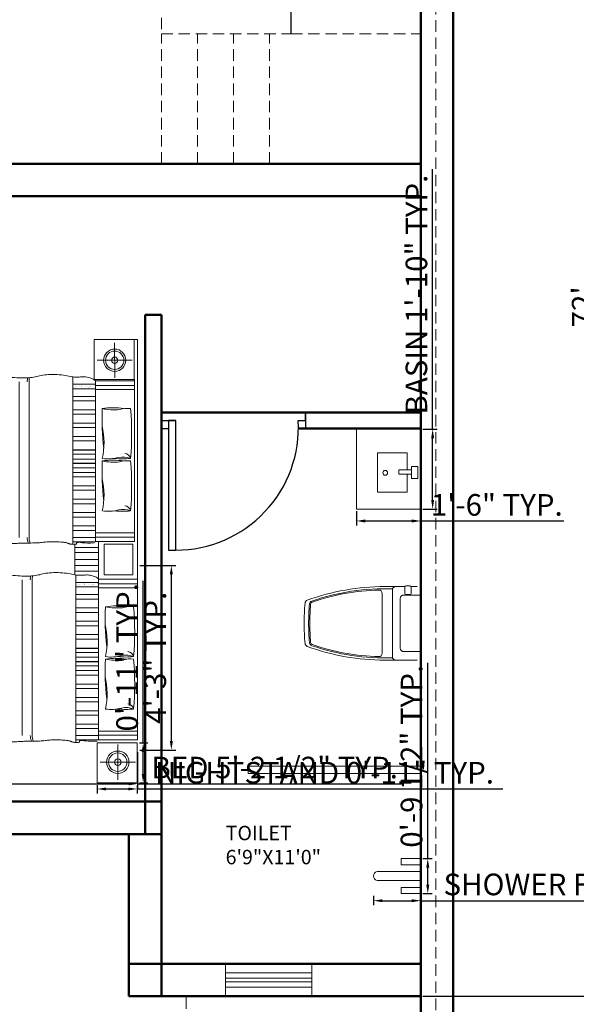
# Model space of a CAD drawing. Units: inches. Extents: x 2123 to 2977, y 1464 to 2698.
# Tile 5 of 10: x 2647 to 2801, y 1923 to 2196. Entities that reach past the tile are written whole.
import ezdxf

# ---------------------------------------------------------------- set-up
doc = ezdxf.new("R2010")
doc.units = ezdxf.units.IN
doc.linetypes.add('HIDDEN2', pattern=[4.7625, 3.175, -1.5875])
for name, color, linetype, lineweight in [('A-ANNO-DIMS', 2, 'Continuous', 18), ('A-AREA-IDEN', 7, 'Continuous', 25), ('A-DOOR', 4, 'Continuous', 25), ('A-FLOR-FIXT', 8, 'Continuous', 20), ('A-FLOR-OVHD', 253, 'HIDDEN2', 18), ('A-FLOR-STRS', 7, 'Continuous', 25), ('A-FLOR-STRS-HIDN', 253, 'HIDDEN2', 18), ('A-FURN', 8, 'Continuous', 18), ('A-FURN-PATT', 252, 'Continuous', 9), ('A-GLAZ', 4, 'Continuous', 18), ('A-WALL', 7, 'Continuous', 50), ('C-PROP', 21, 'HIDDEN2', 18)]:
    doc.layers.add(name, color=color, linetype=linetype, lineweight=lineweight)
doc.styles.get("Standard").update_dxf_attribs({"font": 'arial.ttf'})
doc.dimstyles.new('ISO-25', dxfattribs={"dimtxt": 6, "dimasz": 2.5, "dimexe": 1.25, "dimexo": 0.625, "dimtad": 1, "dimdec": 0, "dimlunit": 3, "dimtxsty": 'Standard', "dimcen": 2.5, "dimadec": 0, "dimazin": 0, "dimtfac": 1, "dimtdec": 0, "dimtmove": 0, "dimatfit": 3, "dimfxl": 1, "dimarcsym": 0})

# ---------------------------------------------------------------- blocks, each defined once
blk = doc.blocks.new('*D9')
at = {"layer": 'A-ANNO-DIMS', "color": 0, "lineweight": -2, "transparency": 16777216}
for p, q in [((2767.56, 2548.37), (2808.58, 2548.37)), ((2807.33, 2545.87), (2807.33, 1686.46)), ((2767.56, 1683.96), (2808.58, 1683.96))]:
    blk.add_line(p, q, dxfattribs=at)
at = {"layer": 'A-ANNO-DIMS', "color": 0, "transparency": 16777216}
for points in [[(2806.91, 2545.87), (2807.74, 2545.87), (2807.33, 2548.37)], [(2806.91, 1686.46), (2807.74, 1686.46), (2807.33, 1683.96)]]:
    blk.add_solid(points, dxfattribs=at)
at = {"layer": 'Defpoints', "color": 0, "transparency": 16777216}
for p in [(2766.94, 2548.37), (2766.94, 1683.96), (2807.33, 1683.96)]:
    blk.add_point(p, dxfattribs=at)
at = {"layer": 'A-ANNO-DIMS', "color": 0, "transparency": 16777216, "insert": (2803.69, 2116.16), "char_height": 6, "attachment_point": 5, "rotation": 90}
blk.add_mtext("72'", dxfattribs=at)
blk = doc.blocks.new('WC-PLAN')
for p, q in [((27.97, 20.42), (22.38, 20.42)), ((24.5, 19.48), (24.5, 10.21)), ((27.93, 20.26), (27.93, 18.53)), ((29.37, 20.57), (28.24, 20.57)), ((31.41, 20.42), (29.65, 20.42)), ((29.69, 20.26), (29.69, 18.53)), ((32.35, 19.48), (32.35, 10.21)), ((21.67, 18.51), (21.67, 10.21)), ((26.7, 17.12), (26.7, 10.21)), ((32.35, 18.06), (27.64, 18.06)), ((29.37, 18.22), (28.24, 18.22)), ((28.24, 18.22), (28.24, 18.06)), ((29.37, 18.22), (29.37, 18.06)), ((21.67, 1.91), (21.67, 10.21)), ((24.5, 0.94), (24.5, 10.21)), ((26.7, 3.3), (26.7, 10.21)), ((32.35, 0.94), (32.35, 10.21)), ((32.35, 2.36), (27.64, 2.36)), ((31.41, 0), (22.38, 0))]:
    blk.add_line(p, q)
for centre, radius, start, end in [((22.38, -42.41), 62.82, 90, 110.0218), ((22.38, -42.41), 62.2, 88.0034, 109.0034), ((22.38, -42.41), 61.88, 91.5459, 109.0034), ((20.73, 18.51), 0.942, 0, 91.5459), ((25.44, 19.48), 0.942, 90, 180), ((28.24, 20.26), 0.314, 150, 180), ((28.24, 20.26), 0.314, 90, 150), ((29.37, 20.26), 0.314, 30, 90), ((29.37, 20.26), 0.314, 0, 30), ((1.19, 15.74), 0.942, 110.0218, 174.8892), ((2.43, 15.51), 0.942, 109.0034, 174.9977), ((27.64, 17.12), 0.942, 90, 180), ((28.24, 18.53), 0.314, 180, 270), ((29.37, 18.53), 0.314, 270, 0), ((62.98, 10.21), 62.98, 174.8892, 180), ((62.98, 10.21), 61.73, 174.9977, 180), ((62.98, 10.21), 61.41, 174.9977, 180), ((2.43, 15.51), 0.628, 109.0034, 174.9977), ((62.98, 10.21), 62.98, 180, 185.1108), ((62.98, 10.21), 61.73, 180, 185.0023), ((62.98, 10.21), 61.41, 180, 185.0023), ((1.19, 4.68), 0.942, 185.1108, 249.9782), ((22.38, 62.82), 62.82, 249.9782, 270), ((2.43, 4.91), 0.942, 185.0023, 250.9966), ((2.43, 4.91), 0.628, 185.0023, 250.9966), ((22.38, 62.82), 62.2, 250.9966, 271.9966), ((22.38, 62.82), 61.88, 250.9966, 268.4541), ((27.64, 3.3), 0.942, 180, 270), ((20.73, 1.91), 0.942, 268.4541, 0), ((25.44, 0.94), 0.942, 180, 270)]:
    blk.add_arc(centre, radius, start, end)
blk = doc.blocks.new('VANITY-BASIN')
blk.add_line((14.09, 15.62), (5.85, 15.62))
for points in [[(0, 22.13), (17.86, 22.13), (17.86, 0), (0, 0)], [(15.3, 11.79), (17.03, 11.79), (17.03, 8.46), (15.3, 8.46)]]:
    blk.add_lwpolyline(points, close=True)
for points in [[(14.09, 9.69), (14.09, 4.64), (5.85, 4.64), (5.85, 15.62)], [(14.09, 15.62), (14.09, 10.87)], [(15.3, 9.69), (11.78, 9.69), (11.78, 10.87), (15.3, 10.87)]]:
    blk.add_lwpolyline(points)
blk.add_circle((8.01, 10.03), 0.665)
blk = doc.blocks.new('SHOWER-FITTING')
for points in [[(7.7, 9.7), (13.11, 9.7), (13.11, 7.96), (7.7, 7.96)], [(7.7, 1.74), (13.11, 1.74), (13.11, 0), (7.7, 0)]]:
    blk.add_lwpolyline(points, close=True)
blk.add_lwpolyline([(1, 6.13), (13.11, 6.13), (13.11, 3.63), (1, 3.63)])
blk.add_arc((1.29, 4.88), 1.29, 102.8146, 257.1854)
blk = doc.blocks.new('BED-WITH-PILLOWS')
for p, q in [((5.75, 4.05), (5.75, 47.2)), ((6.24, 4.05), (6.24, 47.2)), ((10.69, 4.05), (10.69, 47.2)), ((11.18, 4.05), (11.18, 47.2)), ((15.63, 4.05), (15.63, 47.2)), ((16.12, 4.05), (16.12, 47.2)), ((25.45, 4.05), (25.45, 47.2)), ((25.94, 4.05), (25.94, 47.2)), ((30.39, 4.05), (30.39, 47.2)), ((33.11, 4.05), (33.11, 47.2)), ((45.27, 2.11), (45.27, 48.58)), ((51.57, 46.51), (45.27, 46.51)), ((51.57, 45.27), (45.27, 45.27)), ((62.41, 46.17), (51.57, 46.17)), ((62.41, 45.03), (51.57, 45.03)), ((51.57, 28.22), (45.27, 28.22)), ((62.41, 5.26), (51.57, 5.26)), ((62.41, 4.13), (51.57, 4.13)), ((62.41, 2.86), (51.57, 2.86))]:
    blk.add_line(p, q)
for points in [[(51.2, 2.51), (50.14, 2.47), (49.31, 2.46), (48.67, 2.48), (48.19, 2.52), (47.84, 2.56), (47.58, 2.61), (47.39, 2.66), (47.22, 2.69), (47.07, 2.7), (46.91, 2.7), (46.77, 2.68), (46.63, 2.65), (46.51, 2.61), (46.41, 2.56), (46.33, 2.52), (46.28, 2.47), (46.26, 2.42), (46.26, 2.38), (46.28, 2.35), (46.3, 2.31), (46.32, 2.28), (46.32, 2.25), (46.31, 2.22), (46.27, 2.2), (46.19, 2.17), (46.08, 2.15), (45.94, 2.13), (45.78, 2.12), (45.61, 2.11), (45.43, 2.1), (45.25, 2.11), (45.07, 2.12), (44.89, 2.14), (44.73, 2.16), (44.57, 2.2), (44.42, 2.24), (44.28, 2.28), (44.15, 2.32), (44.02, 2.37), (43.89, 2.41), (43.77, 2.46), (43.65, 2.5), (43.51, 2.54), (43.35, 2.58), (43.16, 2.62), (42.93, 2.66), (42.65, 2.69), (42.31, 2.72), (41.91, 2.75), (41.46, 2.78), (40.97, 2.8), (40.46, 2.82), (39.94, 2.82), (39.43, 2.83), (38.94, 2.82), (38.48, 2.81), (38.08, 2.78), (37.71, 2.75), (37.37, 2.71), (37.04, 2.67), (36.71, 2.63), (36.37, 2.59), (36, 2.55), (35.6, 2.52), (35.14, 2.5), (34.65, 2.49), (34.14, 2.48), (33.61, 2.47), (33.1, 2.47), (32.6, 2.47), (32.14, 2.47), (31.72, 2.47), (31.37, 2.46), (31.06, 2.45), (30.79, 2.44), (30.55, 2.42), (30.31, 2.41), (30.08, 2.39), (29.82, 2.38), (29.54, 2.36), (29.21, 2.35), (28.86, 2.33), (28.48, 2.32), (28.09, 2.31), (27.69, 2.3), (27.3, 2.29), (26.93, 2.28), (26.58, 2.27), (26.27, 2.26), (25.99, 2.25), (25.73, 2.24), (25.49, 2.24), (25.25, 2.25), (25.02, 2.27), (24.78, 2.29), (24.53, 2.33), (24.27, 2.38), (23.99, 2.44), (23.7, 2.51), (23.41, 2.57), (23.12, 2.62), (22.85, 2.66), (22.59, 2.69), (22.35, 2.68), (22.13, 2.65), (17.06, 2.6), (16.88, 2.53), (16.71, 2.44), (16.54, 2.35), (16.37, 2.25), (16.2, 2.15), (16.01, 2.05), (15.8, 1.96), (15.58, 1.89), (15.34, 1.82), (15.08, 1.77), (14.81, 1.72), (14.53, 1.69), (14.24, 1.67), (13.93, 1.66), (13.62, 1.66), (13.3, 1.67), (12.98, 1.69), (12.67, 1.72), (12.35, 1.75), (12.05, 1.79), (11.76, 1.84), (11.49, 1.89), (11.24, 1.94), (11, 1.99), (10.76, 2.04), (10.52, 2.09), (10.28, 2.14), (10.02, 2.18), (9.74, 2.21), (9.43, 2.24), (9.08, 2.25), (8.71, 2.26), (8.32, 2.26), (7.93, 2.25), (7.53, 2.24), (7.16, 2.22), (6.8, 2.2), (6.49, 2.17), (6.21, 2.15), (5.97, 2.12), (5.77, 2.09), (5.59, 2.06), (5.44, 2.03), (5.3, 2), (5.18, 1.97), (5.07, 1.94), (4.96, 1.91), (4.85, 1.88), (4.74, 1.85), (4.63, 1.81), (4.51, 1.77), (4.39, 1.72), (4.26, 1.67), (4.12, 1.61), (3.98, 1.53), (3.82, 1.46), (3.67, 1.37), (3.51, 1.27), (3.35, 1.17), (3.19, 1.06), (3.04, 0.94), (2.9, 0.81), (2.76, 0.68), (2.64, 0.54), (2.52, 0.41), (2.4, 0.28), (2.28, 0.18), (2.15, 0.09), (2, 0.03), (1.84, 0), (1.67, 0.01), (1.48, 0.05), (1.28, 0.12), (1.09, 0.21), (0.89, 0.33), (0.71, 0.46), (0.54, 0.6), (0.39, 0.74), (0.26, 0.89), (0.17, 1.04), (0.09, 1.19), (0.04, 1.34), (0.01, 1.49), (0, 1.65), (0.01, 1.81), (0.04, 1.97), (0.08, 2.13), (0.14, 2.3), (0.21, 2.47), (0.29, 2.64), (0.38, 2.82), (0.48, 3), (0.58, 3.18), (0.68, 3.37), (0.79, 3.57), (0.9, 3.77), (1, 3.97), (1.09, 4.19), (1.18, 4.41), (1.26, 4.64), (1.32, 4.89), (1.37, 5.14), (1.4, 5.4), (1.42, 5.68), (1.43, 5.97), (1.43, 6.29), (1.42, 6.62), (1.42, 6.98), (1.41, 7.36), (1.41, 7.77), (1.42, 8.21), (1.44, 8.67), (1.46, 9.16), (1.49, 9.65), (1.52, 10.16), (1.55, 10.68), (1.58, 11.19), (1.61, 11.69), (1.64, 12.19), (1.67, 12.67), (1.69, 13.14), (1.72, 13.6), (1.73, 14.05), (1.75, 14.49), (1.77, 14.91), (1.78, 15.32), (1.79, 15.72), (1.79, 16.1), (1.8, 16.48), (1.81, 16.85), (1.83, 17.21), (1.85, 17.56), (1.88, 17.91), (1.91, 18.25), (1.96, 18.58), (2.01, 18.93), (2.07, 19.29), (2.14, 19.68), (2.21, 20.11), (2.29, 20.58), (2.36, 21.11), (2.44, 21.71), (2.51, 22.39), (2.58, 23.13), (2.64, 23.92), (2.69, 24.77), (2.72, 25.64), (2.73, 26.54), (2.71, 27.44), (2.67, 28.35), (2.59, 24.41), (2.49, 25.28), (2.37, 26.12), (2.24, 26.93), (2.11, 27.7), (1.98, 28.42), (1.86, 29.08), (1.76, 29.68), (1.69, 30.2), (1.64, 30.67), (1.61, 31.08), (1.59, 31.44), (1.59, 31.77), (1.6, 32.08), (1.61, 32.36), (1.63, 32.64), (1.64, 32.92), (1.66, 33.21), (1.67, 33.51), (1.67, 33.82), (1.68, 34.16), (1.68, 34.52), (1.68, 34.92), (1.67, 35.35), (1.66, 35.83), (1.64, 36.35), (1.62, 36.91), (1.61, 37.51), (1.6, 38.16), (1.59, 38.85), (1.59, 39.57), (1.6, 40.34), (1.62, 41.15), (1.65, 41.98), (1.68, 42.82), (1.7, 43.65), (1.72, 44.46), (1.73, 45.24), (1.72, 45.95), (1.7, 46.6), (1.64, 47.17), (1.57, 47.65), (1.48, 48.08), (1.39, 48.45), (1.29, 48.77), (1.19, 49.06), (1.1, 49.32), (1.02, 49.57), (0.96, 49.81), (0.91, 50.04), (0.89, 50.26), (0.87, 50.46), (0.88, 50.65), (0.9, 50.81), (0.93, 50.95), (0.98, 51.06), (1.04, 51.14), (1.12, 51.2), (1.21, 51.22), (1.31, 51.22), (1.43, 51.19), (1.55, 51.15), (1.69, 51.09), (1.84, 51.01), (2.01, 50.92), (2.18, 50.81), (2.36, 50.7), (2.54, 50.57), (2.72, 50.45), (2.91, 50.31), (3.09, 50.18), (3.27, 50.04), (3.45, 49.9), (3.62, 49.77), (3.78, 49.63), (3.93, 49.5), (4.08, 49.37), (4.23, 49.24), (4.37, 49.11), (4.5, 48.99), (4.63, 48.86), (4.76, 48.74), (4.88, 48.62), (5.01, 48.5), (5.14, 48.4), (5.27, 48.3), (5.41, 48.2), (5.55, 48.12), (5.71, 48.05), (5.87, 48), (6.04, 47.95), (6.22, 47.92), (6.39, 47.9), (6.56, 47.89), (6.73, 47.9), (6.89, 47.92), (7.04, 47.96), (7.18, 48.01), (7.31, 48.07), (7.43, 48.13), (7.53, 48.2), (7.61, 48.27), (7.67, 48.33), (7.71, 48.39), (7.73, 48.44), (7.73, 48.49), (7.71, 48.52), (7.68, 48.55), (7.63, 48.58), (7.56, 48.6), (7.49, 48.61), (7.42, 48.62), (7.33, 48.63), (7.25, 48.64), (7.16, 48.64), (7.07, 48.64), (6.99, 48.63), (6.91, 48.62), (6.83, 48.6), (6.77, 48.58), (6.71, 48.55), (6.67, 48.52), (6.63, 48.5), (6.6, 48.47), (6.57, 48.46), (6.56, 48.46), (6.55, 48.48), (6.54, 48.51), (6.54, 48.58)], [(6.54, 48.66), (6.54, 48.76), (6.55, 48.86), (6.56, 48.97), (6.58, 49.08), (6.61, 49.18), (6.63, 49.27), (6.67, 49.34), (6.7, 49.4), (6.75, 49.44), (6.79, 49.47), (6.84, 49.5), (6.9, 49.51), (6.95, 49.52), (7.01, 49.53), (7.07, 49.53), (7.14, 49.53), (7.21, 49.53), (7.28, 49.53), (7.35, 49.53), (7.43, 49.52), (7.51, 49.5), (7.59, 49.49), (7.68, 49.46), (7.77, 49.43), (7.86, 49.4), (7.96, 49.36), (8.06, 49.31), (8.16, 49.26), (8.27, 49.19), (8.37, 49.12), (8.48, 49.04), (8.59, 48.95), (8.69, 48.86), (8.8, 48.76), (8.9, 48.66), (9.01, 48.56), (9.1, 48.45), (9.2, 48.35), (9.29, 48.25), (9.38, 48.16), (9.48, 48.07), (9.61, 48), (9.76, 47.94), (9.95, 47.91), (10.18, 47.89), (10.46, 47.89), (10.81, 47.93), (11.21, 47.98), (11.65, 48.06), (12.15, 48.14), (12.68, 48.23), (13.25, 48.32), (13.84, 48.41), (14.46, 48.49), (15.09, 48.55), (15.74, 48.6), (16.41, 48.64), (17.08, 48.66), (22.63, 48.67), (23.31, 48.67), (23.98, 48.66), (24.65, 48.64), (25.32, 48.61), (25.97, 48.57), (26.62, 48.53), (27.26, 48.49), (27.89, 48.44), (28.51, 48.4), (29.12, 48.36), (29.71, 48.33), (30.3, 48.3), (30.87, 48.28), (31.43, 48.27), (31.97, 48.28), (32.5, 48.29), (33, 48.32), (33.49, 48.36), (33.95, 48.42), (34.39, 48.49), (34.81, 48.58), (35.23, 48.67), (35.64, 48.77), (36.07, 48.87), (36.5, 48.96), (36.96, 49.05), (37.46, 49.12), (37.99, 49.18), (38.55, 49.22), (39.13, 49.24), (39.73, 49.25), (40.33, 49.24), (40.93, 49.22), (41.52, 49.18), (42.1, 49.12), (42.65, 49.05), (43.17, 48.96), (43.66, 48.87), (44.14, 48.78), (44.58, 48.7), (45, 48.62), (45.4, 48.56), (45.77, 48.51), (46.12, 48.5), (46.45, 48.5), (46.77, 48.51), (47.08, 48.53), (47.4, 48.56), (47.73, 48.57), (48.08, 48.58), (48.45, 48.58), (48.84, 48.55), (49.25, 48.49), (49.68, 48.41), (50.1, 48.3), (50.5, 48.16), (50.88, 47.98), (51.23, 47.77), (51.53, 47.52)], [(51.57, 47.43), (51.57, 2.81), (45.27, 2.81)], [(51.57, 47.43), (62.41, 47.43)], [(45.27, 43.15), (51.57, 43.15)], [(51.57, 41.91), (45.27, 41.91)], [(45.27, 39.44), (51.57, 39.44)], [(51.57, 38.2), (45.27, 38.2)], [(45.27, 35.73), (51.57, 35.73)], [(51.57, 34.5), (45.27, 34.5)], [(45.27, 32.03), (51.57, 32.03)], [(51.57, 30.79), (45.27, 30.79)], [(45.27, 28.32), (51.57, 28.32)], [(51.57, 27.09), (45.27, 27.09)], [(45.27, 25.74), (51.57, 25.74)], [(45.27, 24.62), (51.57, 24.62)], [(51.57, 24.51), (45.27, 24.51)], [(51.57, 23.38), (45.27, 23.38)], [(45.27, 22.04), (51.57, 22.04)], [(51.57, 20.8), (45.27, 20.8)], [(45.27, 18.33), (51.57, 18.33)], [(51.57, 17.1), (45.27, 17.1)], [(45.27, 14.63), (51.57, 14.63)], [(51.57, 13.39), (45.27, 13.39)], [(45.27, 10.92), (51.57, 10.92)], [(51.57, 9.69), (45.27, 9.69)], [(45.27, 7.22), (51.57, 7.22)], [(51.57, 5.98), (45.27, 5.98)], [(45.27, 4.05), (51.57, 4.05)]]:
    blk.add_lwpolyline(points)
blk.add_lwpolyline([(51.57, 46.51), (51.57, 45.27), (45.27, 45.27), (45.27, 46.51)], close=True)
for centre, radius, start, end in [((9.74, 47.23), 3.5, 168.8455, 180.4575), ((14.19, 47.23), 3.5, 168.5644, 180.4575), ((14.68, 47.23), 3.5, 167.3874, 180.4575), ((19.13, 47.23), 3.5, 156.778, 180.4575), ((19.62, 47.23), 3.5, 156.3002, 180.4575), ((28.95, 47.23), 3.5, 157.2176, 180.4575), ((29.45, 47.23), 3.5, 157.7219, 180.4575), ((36.12, 47.23), 3.5, 162.3249, 180.4575), ((36.61, 47.23), 3.5, 162.5343, 180.4575), ((113.8, 36.55), 60.42, 176.9417, 187.4263), ((56.43, 21.05), 18.95, 81.0114, 98.9886), ((56.69, 54.69), 15.26, 257.8171, 275.8068), ((60.35, 32.94), 6.89, 82.0225, 107.8578), ((-19.09, 32.85), 80.7, 355.082, 4.918), ((33.93, 30.3), 20.02, 347.406, 13.4182), ((59.54, 25.52), 1.81, 13.0862, 85.1007), ((113.8, 22.01), 60.42, 176.9417, 187.4263), ((55.08, 36.57), 10.76, 261.3968, 285.5408), ((56.43, 6.52), 18.95, 81.0114, 98.9886), ((56.69, 40.15), 15.26, 257.8171, 275.8068), ((59.11, 48.58), 22.76, 264.4677, 275.5323), ((59.18, 20.45), 5.88, 68.7829, 101.9106), ((60.35, 18.41), 6.89, 82.0225, 107.8578), ((-19.09, 18.32), 80.7, 355.082, 4.918), ((33.93, 15.76), 20.02, 347.406, 13.4182), ((55.08, 22.03), 10.76, 261.3968, 285.5408), ((59.11, 34.05), 22.76, 264.4677, 275.5323), ((59.18, 5.91), 5.88, 68.7829, 101.9106), ((59.54, 10.99), 1.81, 13.0862, 85.1007), ((14.19, 4.02), 3.5, 179.5425, 217.0761), ((14.68, 4.02), 3.5, 179.5425, 219.1707), ((19.13, 4.02), 3.5, 179.5425, 212.5319), ((19.62, 4.02), 3.5, 179.5425, 208.4654), ((28.95, 4.02), 3.5, 179.5425, 210.3906), ((29.45, 4.02), 3.5, 179.5425, 210.1306), ((36.12, 4.02), 3.5, 179.5425, 206.8424), ((36.61, 4.02), 3.5, 179.5425, 206.471)]:
    blk.add_arc(centre, radius, start, end)
blk = doc.blocks.new('NIGHTSTAND-WITH-LAMP')
for p, q in [((5.74, 10.64), (5.72, 0.88)), ((0.85, 5.76), (10.61, 5.76))]:
    blk.add_line(p, q)
blk.add_lwpolyline([(11.12, 0), (11.12, 11.12), (0, 11.12), (0, 0)], close=True)
for radius in [3.1, 2.55, 0.89]:
    blk.add_circle((5.73, 5.76), radius)
blk = doc.blocks.new('SHOWER-SCREEN')
for p, q in [((47.94, 2), (0, 2)), ((0, 2), (0, 0)), ((0, 0), (47.94, 0))]:
    blk.add_line(p, q)
blk = doc.blocks.new('*D36')
at = {"layer": 'A-ANNO-DIMS', "color": 0, "lineweight": -2, "transparency": 16777216}
for p, q in [((2761.26, 2082.2), (2761.26, 2154.4)), ((2758.56, 2082.2), (2762.51, 2082.2)), ((2761.26, 2062.56), (2761.26, 2079.7)), ((2758.56, 2060.06), (2762.51, 2060.06))]:
    blk.add_line(p, q, dxfattribs=at)
at = {"layer": 'A-ANNO-DIMS', "color": 0, "transparency": 16777216}
for points in [[(2760.84, 2079.7), (2761.67, 2079.7), (2761.26, 2082.2)], [(2760.84, 2062.56), (2761.67, 2062.56), (2761.26, 2060.06)]]:
    blk.add_solid(points, dxfattribs=at)
at = {"layer": 'Defpoints', "color": 0, "transparency": 16777216}
for p in [(2757.94, 2082.2), (2761.26, 2082.2), (2757.94, 2060.06)]:
    blk.add_point(p, dxfattribs=at)
at = {"layer": 'A-ANNO-DIMS', "color": 0, "transparency": 16777216, "insert": (2757.53, 2119.55), "char_height": 6, "attachment_point": 5, "rotation": 90}
blk.add_mtext('BASIN 1\'-10" TYP.', dxfattribs=at)
blk = doc.blocks.new('*D37')
at = {"layer": 'A-ANNO-DIMS', "color": 0, "lineweight": -2, "transparency": 16777216}
for p, q in [((2740.08, 2059.44), (2740.08, 2055.49)), ((2757.94, 2059.44), (2757.94, 2055.49)), ((2742.58, 2056.74), (2755.44, 2056.74)), ((2757.94, 2056.74), (2797.69, 2056.74))]:
    blk.add_line(p, q, dxfattribs=at)
at = {"layer": 'A-ANNO-DIMS', "color": 0, "transparency": 16777216}
for points in [[(2742.58, 2057.16), (2742.58, 2056.32), (2740.08, 2056.74)], [(2755.44, 2057.16), (2755.44, 2056.32), (2757.94, 2056.74)]]:
    blk.add_solid(points, dxfattribs=at)
at = {"layer": 'Defpoints', "color": 0, "transparency": 16777216}
for p in [(2740.08, 2060.06), (2757.94, 2060.06), (2757.94, 2056.74)]:
    blk.add_point(p, dxfattribs=at)
at = {"layer": 'A-ANNO-DIMS', "color": 0, "transparency": 16777216, "insert": (2779.06, 2060.43), "char_height": 6, "attachment_point": 5}
blk.add_mtext('1\'-6" TYP.', dxfattribs=at)
blk = doc.blocks.new('*D44')
at = {"layer": 'A-ANNO-DIMS', "color": 0, "lineweight": -2, "transparency": 16777216}
for p, q in [((2744.82, 1952.72), (2744.82, 1950.13)), ((2747.32, 1951.38), (2755.44, 1951.38)), ((2757.94, 1952.72), (2757.94, 1950.13)), ((2757.94, 1951.38), (2873.2, 1951.38))]:
    blk.add_line(p, q, dxfattribs=at)
at = {"layer": 'A-ANNO-DIMS', "color": 0, "transparency": 16777216}
for points in [[(2747.32, 1951.79), (2747.32, 1950.96), (2744.82, 1951.38)], [(2755.44, 1951.79), (2755.44, 1950.96), (2757.94, 1951.38)]]:
    blk.add_solid(points, dxfattribs=at)
at = {"layer": 'Defpoints', "color": 0, "transparency": 16777216}
for p in [(2744.82, 1953.34), (2757.94, 1953.34), (2757.94, 1951.38)]:
    blk.add_point(p, dxfattribs=at)
at = {"layer": 'A-ANNO-DIMS', "color": 0, "transparency": 16777216, "insert": (2816.82, 1955.11), "char_height": 6, "attachment_point": 5}
blk.add_mtext('SHOWER FITTING 1\'-1" TYP.', dxfattribs=at)
blk = doc.blocks.new('*D45')
at = {"layer": 'A-ANNO-DIMS', "color": 0, "lineweight": -2, "transparency": 16777216}
for p, q in [((2759.9, 1963.04), (2759.9, 2017.35)), ((2758.56, 1963.04), (2761.15, 1963.04)), ((2759.9, 1955.84), (2759.9, 1960.54)), ((2758.56, 1953.34), (2761.15, 1953.34))]:
    blk.add_line(p, q, dxfattribs=at)
at = {"layer": 'A-ANNO-DIMS', "color": 0, "transparency": 16777216}
for points in [[(2759.49, 1960.54), (2760.32, 1960.54), (2759.9, 1963.04)], [(2759.49, 1955.84), (2760.32, 1955.84), (2759.9, 1953.34)]]:
    blk.add_solid(points, dxfattribs=at)
at = {"layer": 'Defpoints', "color": 0, "transparency": 16777216}
for p in [(2757.94, 1963.04), (2759.9, 1963.04), (2757.94, 1953.34)]:
    blk.add_point(p, dxfattribs=at)
at = {"layer": 'A-ANNO-DIMS', "color": 0, "transparency": 16777216, "insert": (2756.17, 1991.45), "char_height": 6, "attachment_point": 5, "rotation": 90}
blk.add_mtext('0\'-9 1/2" TYP.', dxfattribs=at)
blk = doc.blocks.new('*D48')
at = {"layer": 'A-ANNO-DIMS', "color": 0, "lineweight": -2, "transparency": 16777216}
for p, q in [((2616.93, 1992.55), (2616.93, 1982.56)), ((2679.35, 1992.55), (2679.35, 1982.56)), ((2619.43, 1983.81), (2676.85, 1983.81)), ((2679.35, 1983.81), (2752.95, 1983.81))]:
    blk.add_line(p, q, dxfattribs=at)
at = {"layer": 'A-ANNO-DIMS', "color": 0, "transparency": 16777216}
for points in [[(2619.43, 1984.23), (2619.43, 1983.39), (2616.93, 1983.81)], [(2676.85, 1984.23), (2676.85, 1983.39), (2679.35, 1983.81)]]:
    blk.add_solid(points, dxfattribs=at)
at = {"layer": 'Defpoints', "color": 0, "transparency": 16777216}
for p in [(2616.93, 1993.17), (2679.35, 1993.17), (2679.35, 1983.81)]:
    blk.add_point(p, dxfattribs=at)
at = {"layer": 'A-ANNO-DIMS', "color": 0, "transparency": 16777216, "insert": (2717.4, 1987.54), "char_height": 6, "attachment_point": 5}
blk.add_mtext('BED 5\'-2 1/2" TYP.', dxfattribs=at)
blk = doc.blocks.new('*D49')
at = {"layer": 'A-ANNO-DIMS', "color": 0, "lineweight": -2, "transparency": 16777216}
for p, q in [((2679.97, 2044.39), (2689.96, 2044.39)), ((2688.71, 1995.67), (2688.71, 2041.89)), ((2679.97, 1993.17), (2689.96, 1993.17))]:
    blk.add_line(p, q, dxfattribs=at)
at = {"layer": 'A-ANNO-DIMS', "color": 0, "transparency": 16777216}
for points in [[(2688.29, 2041.89), (2689.13, 2041.89), (2688.71, 2044.39)], [(2688.29, 1995.67), (2689.13, 1995.67), (2688.71, 1993.17)]]:
    blk.add_solid(points, dxfattribs=at)
at = {"layer": 'Defpoints', "color": 0, "transparency": 16777216}
for p in [(2679.35, 2044.39), (2688.71, 2044.39), (2679.35, 1993.17)]:
    blk.add_point(p, dxfattribs=at)
at = {"layer": 'A-ANNO-DIMS', "color": 0, "transparency": 16777216, "insert": (2685.02, 2018.78), "char_height": 6, "attachment_point": 5, "rotation": 90}
blk.add_mtext('4\'-3" TYP.', dxfattribs=at)
blk = doc.blocks.new('*D50')
at = {"layer": 'A-ANNO-DIMS', "color": 0, "lineweight": -2, "transparency": 16777216}
for p, q in [((2668.11, 1983.42), (2668.11, 1981.13)), ((2670.61, 1982.38), (2676.73, 1982.38)), ((2679.23, 1983.42), (2679.23, 1981.13)), ((2679.23, 1982.38), (2780.73, 1982.38))]:
    blk.add_line(p, q, dxfattribs=at)
at = {"layer": 'A-ANNO-DIMS', "color": 0, "transparency": 16777216}
for points in [[(2670.61, 1982.8), (2670.61, 1981.96), (2668.11, 1982.38)], [(2676.73, 1982.8), (2676.73, 1981.96), (2679.23, 1982.38)]]:
    blk.add_solid(points, dxfattribs=at)
at = {"layer": 'Defpoints', "color": 0, "transparency": 16777216}
for p in [(2668.11, 1984.05), (2679.23, 1984.05), (2679.23, 1982.38)]:
    blk.add_point(p, dxfattribs=at)
at = {"layer": 'A-ANNO-DIMS', "color": 0, "transparency": 16777216, "insert": (2731.23, 1986.11), "char_height": 6, "attachment_point": 5}
blk.add_mtext('NIGHTSTAND 0\'-11" TYP.', dxfattribs=at)
blk = doc.blocks.new('*D51')
at = {"layer": 'A-ANNO-DIMS', "color": 0, "lineweight": -2, "transparency": 16777216}
for p, q in [((2680.89, 1995.17), (2680.89, 2040.15)), ((2679.85, 1995.17), (2682.14, 1995.17)), ((2680.89, 1986.55), (2680.89, 1992.67)), ((2679.85, 1984.05), (2682.14, 1984.05))]:
    blk.add_line(p, q, dxfattribs=at)
at = {"layer": 'A-ANNO-DIMS', "color": 0, "transparency": 16777216}
for points in [[(2680.48, 1992.67), (2681.31, 1992.67), (2680.89, 1995.17)], [(2680.48, 1986.55), (2681.31, 1986.55), (2680.89, 1984.05)]]:
    blk.add_solid(points, dxfattribs=at)
at = {"layer": 'Defpoints', "color": 0, "transparency": 16777216}
for p in [(2679.23, 1995.17), (2680.89, 1995.17), (2679.23, 1984.05)]:
    blk.add_point(p, dxfattribs=at)
at = {"layer": 'A-ANNO-DIMS', "color": 0, "transparency": 16777216, "insert": (2677.2, 2018.91), "char_height": 6, "attachment_point": 5, "rotation": 90}
blk.add_mtext('0\'-11" TYP.', dxfattribs=at)
blk = doc.blocks.new('*D55')
at = {"layer": 'A-ANNO-DIMS', "color": 0, "lineweight": -2, "transparency": 16777216}
for p, q in [((2758.56, 1924.87), (2820.89, 1924.87)), ((2819.64, 1695.76), (2819.64, 1922.37)), ((2758.56, 1693.26), (2820.89, 1693.26))]:
    blk.add_line(p, q, dxfattribs=at)
at = {"layer": 'A-ANNO-DIMS', "color": 0, "transparency": 16777216}
for points in [[(2819.22, 1922.37), (2820.05, 1922.37), (2819.64, 1924.87)], [(2819.22, 1695.76), (2820.05, 1695.76), (2819.64, 1693.26)]]:
    blk.add_solid(points, dxfattribs=at)
at = {"layer": 'Defpoints', "color": 0, "transparency": 16777216}
for p in [(2757.94, 1924.87), (2819.64, 1924.87), (2757.94, 1693.26)]:
    blk.add_point(p, dxfattribs=at)
at = {"layer": 'A-ANNO-DIMS', "color": 0, "transparency": 16777216, "insert": (2815.91, 1809.06), "char_height": 6, "attachment_point": 5, "rotation": 90}
blk.add_mtext('19\'-3 1/2"', dxfattribs=at)
blk = doc.blocks.new('*D57')
at = {"layer": 'A-ANNO-DIMS', "color": 0, "lineweight": -2, "transparency": 16777216}
for p, q in [((2555.89, 1805.13), (2555.89, 2606.82)), ((2757.94, 1805.13), (2757.94, 2606.82)), ((2558.39, 2605.57), (2755.44, 2605.57))]:
    blk.add_line(p, q, dxfattribs=at)
at = {"layer": 'A-ANNO-DIMS', "color": 0, "transparency": 16777216}
for points in [[(2558.39, 2605.99), (2558.39, 2605.15), (2555.89, 2605.57)], [(2755.44, 2605.99), (2755.44, 2605.15), (2757.94, 2605.57)]]:
    blk.add_solid(points, dxfattribs=at)
at = {"layer": 'Defpoints', "color": 0, "transparency": 16777216}
for p in [(2757.94, 2605.57), (2555.89, 1804.5), (2757.94, 1804.5)]:
    blk.add_point(p, dxfattribs=at)
at = {"layer": 'A-ANNO-DIMS', "color": 0, "transparency": 16777216, "insert": (2656.91, 2609.26), "char_height": 6, "attachment_point": 5}
blk.add_mtext('16\'-10"', dxfattribs=at)

msp = doc.modelspace()

# ---------------------------------------------------------------- hatches: boundary and pattern name
at = {"layer": 'A-FURN-PATT'}
h = msp.add_hatch(dxfattribs=at)
h.set_pattern_fill('AR-SAND', color=256, scale=0.673778, angle=1350, style=0)
h.set_pattern_definition([(307.5, (1997.5053, 3855.3914), (1.2982516, 0.04244354), [0, -1.0241427, 0, -1.14542274, 0, -1.0948894]), (277.5, (1997.5053, 3855.3914), (1.9015002, -1.1924368), [0, -0.552498, 0, -0.923076, 0, -0.3537335]), (237.5, (1997.5053, 3856.2201), (0.00381295, -2.0982405), [0, -0.33688904, 0, -1.21280055, 0, -1.5833785]), (227.5, (1997.5053, 3856.2201), (0.5913586, -2.0254622), [0, -0.1684445, 0, -0.79505814, 0, -0.9096004])])
h.paths.add_polyline_path([(2667.64, 2094.66), (2667.64, 2093.43), (2661.35, 2093.43), (2661.35, 2094.66)])
h = msp.add_hatch(dxfattribs=at)
h.set_pattern_fill('AR-SAND', color=256, scale=0.673778, angle=1350, style=0)
h.set_pattern_definition([(307.5, (1998.3629, 3800.4087), (1.2982516, 0.04244354), [0, -1.0241427, 0, -1.14542274, 0, -1.0948894]), (277.5, (1998.3629, 3800.4087), (1.9015002, -1.1924368), [0, -0.552498, 0, -0.923076, 0, -0.3537335]), (237.5, (1998.3629, 3801.2375), (0.00381295, -2.0982405), [0, -0.33688904, 0, -1.21280055, 0, -1.5833785]), (227.5, (1998.3629, 3801.2375), (0.5913586, -2.0254622), [0, -0.1684445, 0, -0.79505814, 0, -0.9096004])])
h.paths.add_polyline_path([(2668.5, 2039.68), (2668.5, 2038.45), (2662.2, 2038.45), (2662.2, 2039.68)])

# ---------------------------------------------------------------- linework, layer by layer
at = {"layer": 'A-DOOR'}
for p, q in [((2685.94, 2084.65), (2685.94, 2084.65)), ((2685.94, 2084.65), (2687.94, 2084.65)), ((2687.94, 2084.65), (2687.94, 2048.65)), ((2689.94, 2084.65), (2687.94, 2084.65)), ((2687.94, 2084.65), (2689.94, 2084.65)), ((2689.94, 2048.65), (2689.94, 2084.65)), ((2723.94, 2084.65), (2725.94, 2084.65)), ((2725.94, 2084.65), (2725.94, 2086.87)), ((2725.94, 2086.87), (2725.94, 2082.37)), ((2685.94, 2082.37), (2687.94, 2082.37)), ((2687.94, 2048.65), (2689.94, 2048.65))]:
    msp.add_line(p, q, dxfattribs=at)
msp.add_arc((2689.94, 2082.71), 34.06, 270, 3.2732, dxfattribs=at)
at = {"layer": 'A-FLOR-OVHD'}
msp.add_line((2692.84, 1892.82), (2692.84, 1924.87), dxfattribs=at)
at = {"layer": 'A-FLOR-STRS'}
msp.add_line((2721.94, 2191.87), (2721.94, 2231.87), dxfattribs=at)
at = {"layer": 'A-FLOR-STRS-HIDN'}
for p, q in [((2685.94, 2286.87), (2685.94, 2191.87)), ((2685.94, 2155.87), (2685.94, 2191.87)), ((2685.94, 2191.87), (2721.94, 2191.87)), ((2695.94, 2155.87), (2695.94, 2191.87)), ((2705.94, 2155.87), (2705.94, 2191.87)), ((2715.94, 2155.87), (2715.94, 2191.87)), ((2721.94, 2191.87), (2757.94, 2191.87))]:
    msp.add_line(p, q, dxfattribs=at)
at = {"layer": 'A-FURN'}
for p, q in [((2679.35, 2107.13), (2678.37, 2107.13)), ((2679.35, 2040.61), (2679.35, 2107.13)), ((2678.49, 2051.01), (2678.49, 2095.98)), ((2681.44, 2095.72), (2681.44, 2051.15)), ((2661.93, 2041.79), (2661.94, 2050.28)), ((2661.94, 2049.35), (2668.5, 2049.35)), ((2668.5, 2040.61), (2668.5, 2051.01)), ((2661.94, 2047.98), (2668.5, 2047.98)), ((2661.94, 2046.04), (2668.5, 2046.04)), ((2661.94, 2044.35), (2668.5, 2044.35)), ((2661.93, 2042.78), (2668.5, 2042.78)), ((2679.35, 2040.61), (2679.35, 1996.03))]:
    msp.add_line(p, q, dxfattribs=at)
msp.add_lwpolyline([(2670.07, 2050.26), (2678.05, 2050.26), (2678.05, 2041.77), (2670.07, 2041.77)], close=True, dxfattribs=at)
at = {"layer": 'A-GLAZ'}
for p, q in [((2703.75, 1933.87), (2703.75, 1924.87)), ((2727.75, 1929.37), (2727.75, 1933.87)), ((2727.75, 1933.87), (2727.75, 1924.87)), ((2703.75, 1931.37), (2727.75, 1931.37)), ((2703.75, 1929.87), (2727.75, 1929.87)), ((2703.75, 1924.87), (2703.75, 1929.37)), ((2703.75, 1928.87), (2727.75, 1928.87)), ((2703.75, 1927.37), (2727.75, 1927.37))]:
    msp.add_line(p, q, dxfattribs=at)
at = {"layer": 'A-WALL'}
for p, q in [((2766.94, 2425.87), (2766.94, 1897.87)), ((2757.94, 2416.87), (2757.94, 1897.87)), ((2580.79, 2155.87), (2757.94, 2155.87)), ((2580.79, 2146.87), (2757.94, 2146.87)), ((2681.44, 2086.87), (2681.44, 2113.91)), ((2681.44, 2113.91), (2685.94, 2113.91)), ((2685.94, 2113.91), (2685.94, 2086.87)), ((2681.44, 2086.87), (2681.44, 1969.87)), ((2685.94, 2086.87), (2757.94, 2086.87)), ((2685.94, 2086.87), (2685.94, 1924.87)), ((2723.99, 2082.37), (2757.94, 2082.37)), ((2456.44, 1978.87), (2685.94, 1978.87)), ((2447.44, 1969.87), (2685.94, 1969.87)), ((2676.94, 1969.87), (2676.94, 1924.87)), ((2676.94, 1933.87), (2757.94, 1933.87)), ((2676.94, 1924.87), (2757.94, 1924.87))]:
    msp.add_line(p, q, dxfattribs=at)
msp.add_lwpolyline([(2757.94, 2086.87), (2757.94, 2086.7)], dxfattribs=at)
at = {"layer": 'C-PROP'}
msp.add_line((2762.16, 2552.87), (2762.16, 1683.96), dxfattribs=at)

# ---------------------------------------------------------------- block references
at = {"layer": 'A-FLOR-FIXT'}
for name, p in [('VANITY-BASIN', (2740.08, 2060.06)), ('WC-PLAN', (2725.58, 2018.13)), ('SHOWER-SCREEN', (2710, 1986.69)), ('SHOWER-FITTING', (2744.82, 1953.34))]:
    msp.add_blockref(name, p, dxfattribs=at)
at = {"layer": 'A-FURN', "extrusion": (0, 0, -1), "zscale": -1, "rotation": 180}
msp.add_blockref('NIGHTSTAND-WITH-LAMP', (-2667.25, 2107.09), dxfattribs=at)
at = {"layer": 'A-FURN'}
for name, p in [('BED-WITH-PILLOWS', (2616.08, 2048.15)), ('BED-WITH-PILLOWS', (2616.93, 1993.17)), ('NIGHTSTAND-WITH-LAMP', (2668.11, 1984.05))]:
    msp.add_blockref(name, p, dxfattribs=at)

# ---------------------------------------------------------------- texts
at = {"layer": 'A-AREA-IDEN', "insert": (2703.78, 1972.15), "char_height": 4, "attachment_point": 1}
msp.add_mtext_dynamic_manual_height_columns('TOILET\\P6\'9"X11\'0"', width=166.3871, gutter_width=12.5, heights=[0], dxfattribs=at)

# ---------------------------------------------------------------- dimensions: what is measured, and where the dimension line sits
at = {"layer": 'A-ANNO-DIMS'}
dim = msp.add_linear_dim(base=(2757.9353, 2605.5708), p1=(2555.8869, 1804.5032), p2=(2757.9353, 1804.5032), dimstyle='ISO-25', override={"dimdec": 1, "dimlfac": 1, "dimrnd": 0, "dimzin": 1, "dimdsep": 46, "dimlunit": 4, "dimfrac": 2}, dxfattribs=at)
dim.commit()
dim.dimension.update_dxf_attribs({"geometry": '*D57', "text_midpoint": (2656.9111, 2609.2592)})
for base, p1, p2, override, picture, middle in [((2807.33, 1683.96), (2766.94, 2548.37), (2766.94, 1683.96), {"dimclrd": 0, "dimclre": 0, "dimclrt": 0}, '*D9', (2803.69, 2116.16)), ((2819.64, 1924.87), (2757.94, 1693.26), (2757.94, 1924.87), {"dimdec": 1, "dimlfac": 1, "dimrnd": 0, "dimzin": 1, "dimdsep": 46, "dimlunit": 4, "dimfrac": 2}, '*D55', (2815.91, 1809.06))]:
    dim = msp.add_linear_dim(base=base, p1=p1, p2=p2, angle=90, dimstyle='ISO-25', override=override, dxfattribs=at)
    dim.commit()
    dim.dimension.update_dxf_attribs({"geometry": picture, "text_midpoint": middle})
for base, p1, p2, text, picture, middle in [((2761.26, 2082.2), (2757.94, 2060.06), (2757.94, 2082.2), 'BASIN <> TYP.', '*D36', (2757.53, 2119.55)), ((2688.71, 2044.39), (2679.35, 1993.17), (2679.35, 2044.39), '<> TYP.', '*D49', (2685.02, 2018.78)), ((2680.89, 1995.17), (2679.23, 1984.05), (2679.23, 1995.17), '<> TYP.', '*D51', (2677.2, 2018.91)), ((2759.9, 1963.04), (2757.94, 1953.34), (2757.94, 1963.04), '<> TYP.', '*D45', (2756.17, 1991.45))]:
    dim = msp.add_linear_dim(base=base, p1=p1, p2=p2, angle=90, text=text, dimstyle='ISO-25', override={"dimdec": 1, "dimlfac": 1, "dimrnd": 0, "dimzin": 1, "dimdsep": 46, "dimlunit": 4, "dimfrac": 2}, dxfattribs=at)
    dim.commit()
    dim.dimension.update_dxf_attribs({"geometry": picture, "text_midpoint": middle})
for base, p1, p2, text, picture, middle in [((2757.94, 2056.74), (2740.08, 2060.06), (2757.94, 2060.06), '<> TYP.', '*D37', (2779.06, 2060.43)), ((2679.35, 1983.81), (2616.93, 1993.17), (2679.35, 1993.17), 'BED <> TYP.', '*D48', (2717.4, 1987.54)), ((2679.23, 1982.38), (2668.11, 1984.05), (2679.23, 1984.05), 'NIGHTSTAND <> TYP.', '*D50', (2731.23, 1986.11)), ((2757.94, 1951.38), (2744.82, 1953.34), (2757.94, 1953.34), 'SHOWER FITTING <> TYP.', '*D44', (2816.82, 1955.11))]:
    dim = msp.add_linear_dim(base=base, p1=p1, p2=p2, text=text, dimstyle='ISO-25', override={"dimdec": 1, "dimlfac": 1, "dimrnd": 0, "dimzin": 1, "dimdsep": 46, "dimlunit": 4, "dimfrac": 2}, dxfattribs=at)
    dim.commit()
    dim.dimension.update_dxf_attribs({"geometry": picture, "text_midpoint": middle})

doc.saveas('drawing.dxf')
